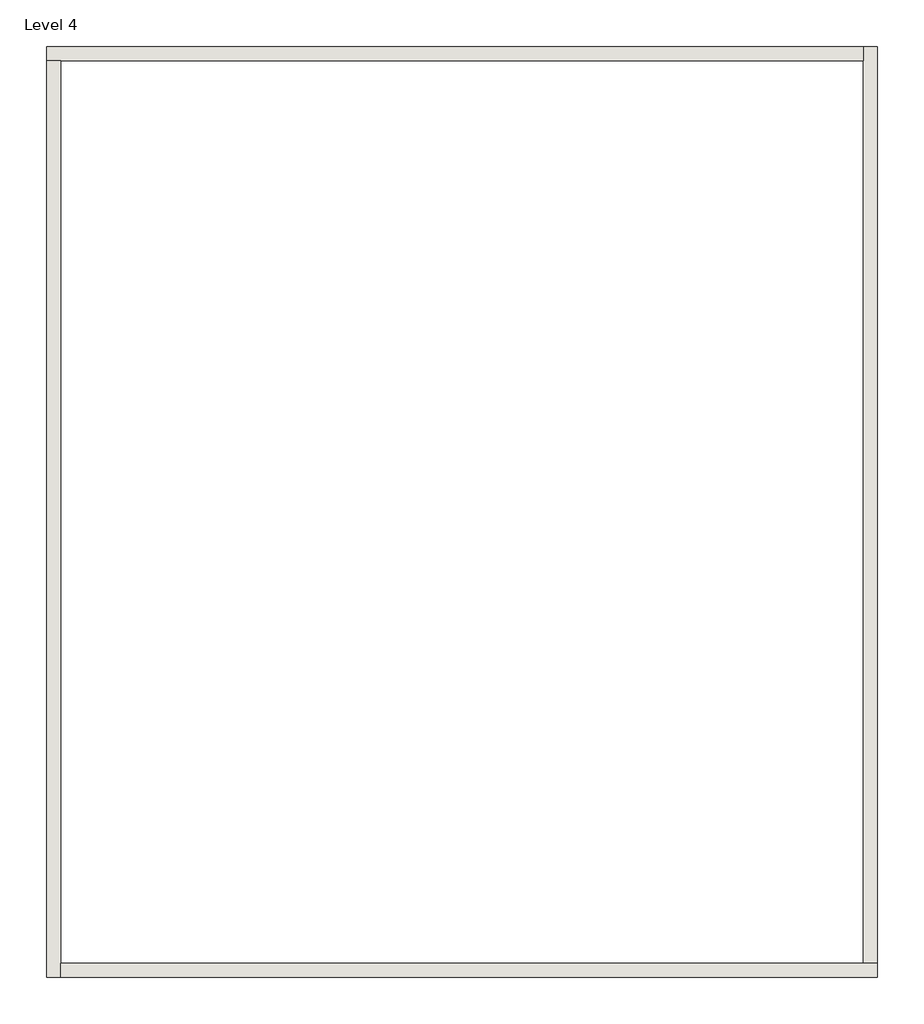
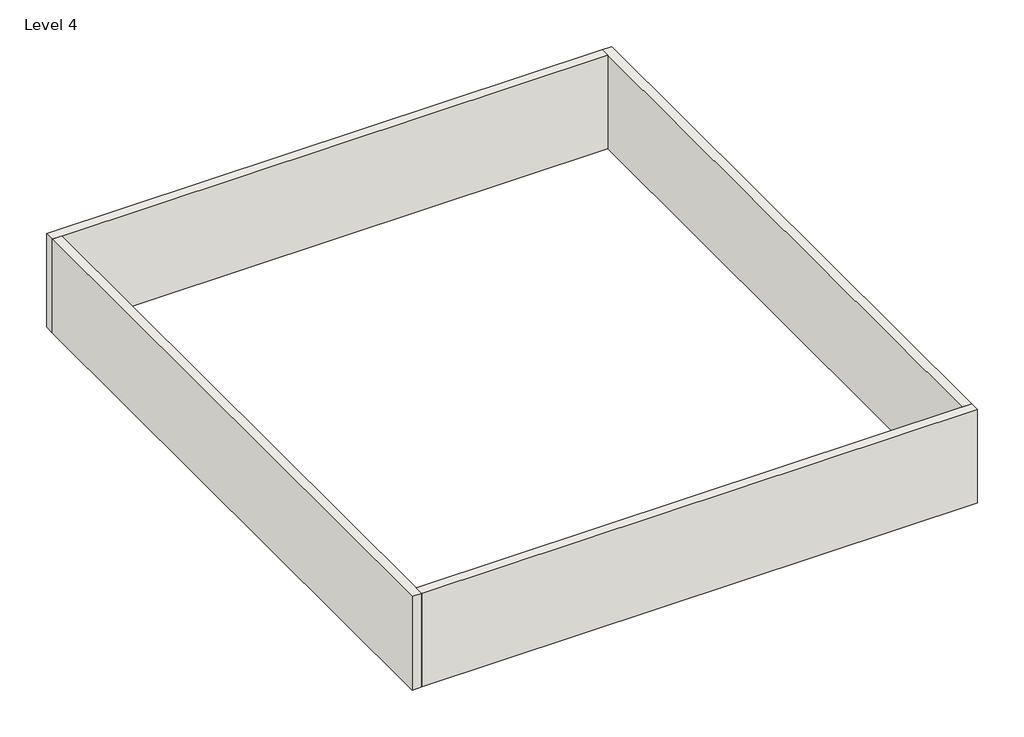
# One storey: 4 walls.
"""IFC4 building model written with IfcOpenShell, lengths in millimetres."""

from ifc_helpers import new_model, si_unit, origin, place, context, project, spatial, faceted_brep, element, save

model = new_model("IFC4")

# Units and contexts
model_context = context("Model", 3, world=origin())
ifc_project = project(units=[si_unit("LENGTHUNIT", "METRE", prefix="MILLI")], contexts=[model_context])

# Site, building, storey
site = spatial("IfcSite", under=ifc_project)
building = spatial("IfcBuilding", under=site)
storey = spatial("IfcBuildingStorey", under=building, Name="Level 4", Elevation=6858.0)

# Walls
placement = place(None, origin())
element("IfcWall", 1, ObjectType="4\"", at=placement, inside=storey, context=model_context, shape_type="Brep", body=[
    faceted_brep([(-2417.9243879, -3041.7883122, 6858.0), (-2519.5243879, -3041.7883122, 6858.0), (-8259.9243879, -3041.7883122, 6858.0), (-8259.9243879, -3041.7883122, 7899.4), (-2519.5243879, -3041.7883122, 7899.4), (-2417.9243879, -3041.7883122, 7899.4), (-2417.9243879, -3143.3883122, 6858.0), (-2417.9243879, -3143.3883122, 7899.4), (-8259.9243879, -3143.3883122, 7899.4), (-8259.9243879, -3143.3883122, 6858.0)], [[[0, 1, 2, 3, 4, 5]], [[6, 7, 8, 9]], [[2, 1, 0, 6, 9]], [[5, 4, 3, 8, 7]], [[0, 5, 7, 6]], [[3, 2, 9, 8]]]),
])
element("IfcWall", 2, ObjectType="4\"", at=placement, inside=storey, context=model_context, shape_type="Brep", body=[
    faceted_brep([(-2519.5243879, 3511.4116878, 6858.0), (-2519.5243879, 3409.8116878, 6858.0), (-2519.5243879, -3041.7883122, 6858.0), (-2519.5243879, -3041.7883122, 7899.4), (-2519.5243879, 3409.8116878, 7899.4), (-2519.5243879, 3511.4116878, 7899.4), (-2417.9243879, 3511.4116878, 6858.0), (-2417.9243879, 3511.4116878, 7899.4), (-2417.9243879, -3041.7883122, 7899.4), (-2417.9243879, -3041.7883122, 6858.0)], [[[0, 1, 2, 3, 4, 5]], [[6, 7, 8, 9]], [[2, 1, 0, 6, 9]], [[5, 4, 3, 8, 7]], [[0, 5, 7, 6]], [[3, 2, 9, 8]]]),
])
element("IfcWall", 3, ObjectType="4\"", at=placement, inside=storey, context=model_context, shape_type="Brep", body=[
    faceted_brep([(-8361.5243879, 3409.8116878, 6858.0), (-8259.9243879, 3409.8116878, 6858.0), (-2519.5243879, 3409.8116878, 6858.0), (-2519.5243879, 3409.8116878, 7899.4), (-8259.9243879, 3409.8116878, 7899.4), (-8361.5243879, 3409.8116878, 7899.4), (-8361.5243879, 3511.4116878, 6858.0), (-8361.5243879, 3511.4116878, 7899.4), (-2519.5243879, 3511.4116878, 7899.4), (-2519.5243879, 3511.4116878, 6858.0)], [[[0, 1, 2, 3, 4, 5]], [[6, 7, 8, 9]], [[2, 1, 0, 6, 9]], [[5, 4, 3, 8, 7]], [[0, 5, 7, 6]], [[3, 2, 9, 8]]]),
])
element("IfcWall", 4, ObjectType="4\"", at=placement, inside=storey, context=model_context, shape_type="Brep", body=[
    faceted_brep([(-8259.9243879, -3143.3883122, 6858.0), (-8259.9243879, -3041.7883122, 6858.0), (-8259.9243879, 3409.8116878, 6858.0), (-8259.9243879, 3409.8116878, 7899.4), (-8259.9243879, -3041.7883122, 7899.4), (-8259.9243879, -3143.3883122, 7899.4), (-8361.5243879, -3143.3883122, 6858.0), (-8361.5243879, -3143.3883122, 7899.4), (-8361.5243879, 3409.8116878, 7899.4), (-8361.5243879, 3409.8116878, 6858.0)], [[[0, 1, 2, 3, 4, 5]], [[6, 7, 8, 9]], [[2, 1, 0, 6, 9]], [[5, 4, 3, 8, 7]], [[0, 5, 7, 6]], [[3, 2, 9, 8]]]),
])

save(model, "model.ifc")

# Revit data of these elements
# Type "4\""
#   Assembly Code = "B2010"
# Elements 1, 2, 3, 4 (IfcWall, "4\"")
#   Top Offset = 0' - 0"
#   Base Offset = 0' - 0"
#   wall height = 3' - 5"
#   Phase Created = New Construction
#   Base Constraint = Level 4
#   Top Constraint = Level 5
